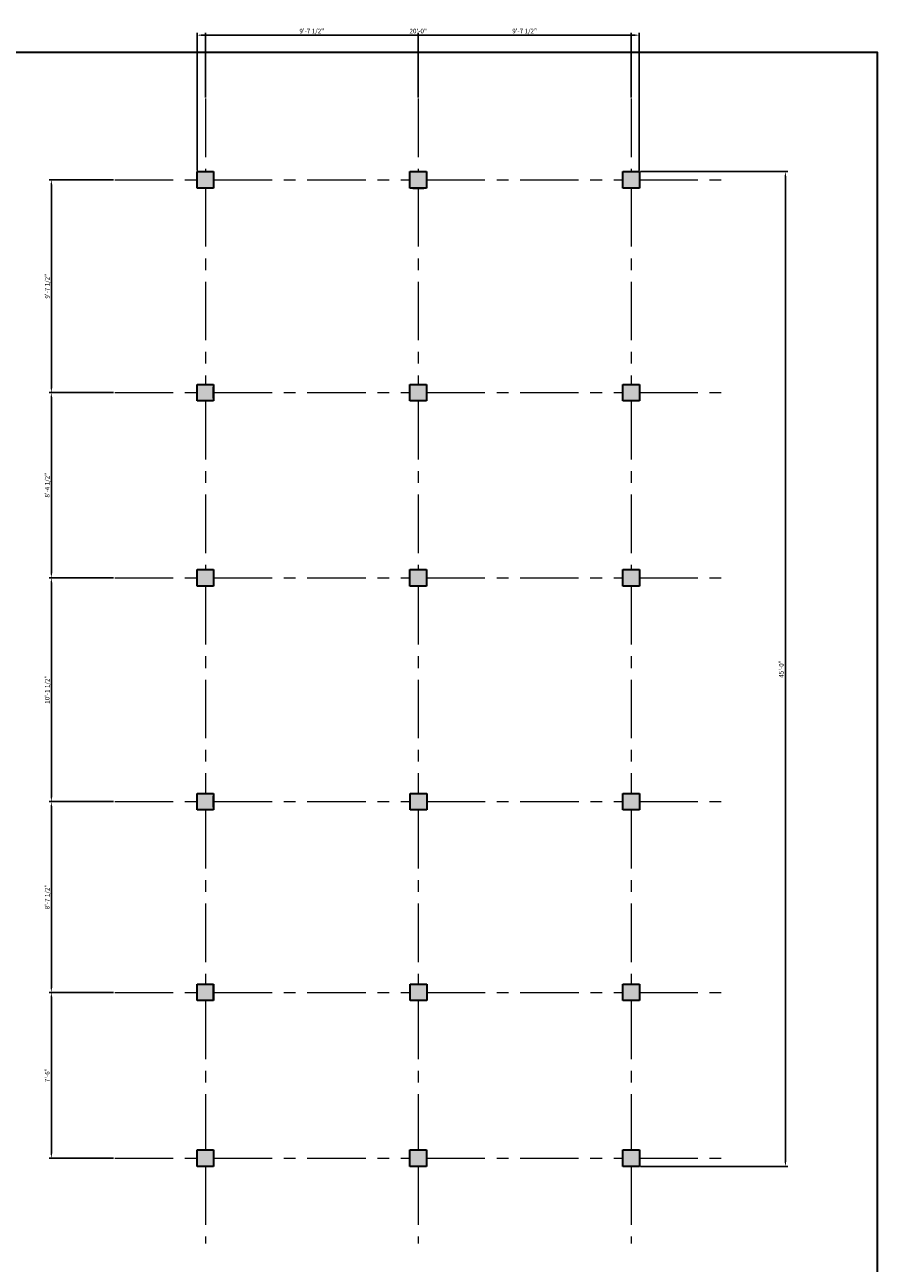
# Model space of a CAD drawing. Units: inches. Extents: x 2150 to 10686, y 1035 to 5077.
# Tile 12 of 12: x 10224 to 10686, y 1433 to 2106. Entities that reach past the tile are written whole.
import ezdxf

# ---------------------------------------------------------------- set-up
doc = ezdxf.new("R2010")
doc.units = ezdxf.units.IN
doc.linetypes.add('CENTER', pattern=[50.8, 31.75, -6.35, 6.35, -6.35])
for name, color, linetype, lineweight in [('A-ANNO-DIMS', 2, 'Continuous', 18), ('A-ANNO-TTLB', 7, 'Continuous', 35), ('A-COLS', 7, 'Continuous', 35), ('A-COLS-PATT', 8, 'Continuous', 13), ('A-GRID', 1, 'CENTER', 18)]:
    doc.layers.add(name, color=color, linetype=linetype, lineweight=lineweight)
doc.styles.get("Standard").update_dxf_attribs({"font": 'arial.ttf'})
doc.dimstyles.new('ISO-25', dxfattribs={"dimtxt": 2.5, "dimasz": 2.5, "dimexe": 1.25, "dimexo": 0.625, "dimtad": 1, "dimdec": 0, "dimlunit": 3, "dimtxsty": 'Standard', "dimcen": 2.5, "dimadec": 0, "dimazin": 0, "dimtfac": 1, "dimtdec": 0, "dimtmove": 0, "dimatfit": 3, "dimfxl": 1, "dimarcsym": 0})

# ---------------------------------------------------------------- blocks, each defined once
blk = doc.blocks.new('COL-SQUARE-9IN')
for p, q in [((0, 9), (9, 9)), ((0, 0), (0, 9)), ((9, 9), (9, 0)), ((9, 0), (0, 0))]:
    blk.add_line(p, q)
blk = doc.blocks.new('*D86')
at = {"layer": 'A-ANNO-DIMS', "color": 0, "lineweight": -2, "transparency": 16777216}
for p, q in [((10321.75, 2066.22), (10321.75, 2101.24)), ((10324.25, 2099.99), (10434.75, 2099.99)), ((10437.25, 2066.22), (10437.25, 2101.24))]:
    blk.add_line(p, q, dxfattribs=at)
at = {"layer": 'A-ANNO-DIMS', "color": 0, "transparency": 16777216}
for points in [[(10324.25, 2100.41), (10324.25, 2099.57), (10321.75, 2099.99)], [(10434.75, 2100.41), (10434.75, 2099.57), (10437.25, 2099.99)]]:
    blk.add_solid(points, dxfattribs=at)
at = {"layer": 'Defpoints', "color": 0, "transparency": 16777216}
for p in [(10437.25, 2099.99), (10321.75, 2065.59), (10437.25, 2065.59)]:
    blk.add_point(p, dxfattribs=at)
at = {"layer": 'A-ANNO-DIMS', "color": 0, "transparency": 16777216, "insert": (10379.5, 2101.91), "char_height": 2.5, "attachment_point": 5}
blk.add_mtext('9\'-7 1/2"', dxfattribs=at)
blk = doc.blocks.new('*D87')
at = {"layer": 'A-ANNO-DIMS', "color": 0, "lineweight": -2, "transparency": 16777216}
for p, q in [((10437.25, 2066.22), (10437.25, 2101.24)), ((10439.75, 2099.99), (10550.25, 2099.99)), ((10552.75, 2066.22), (10552.75, 2101.24))]:
    blk.add_line(p, q, dxfattribs=at)
at = {"layer": 'A-ANNO-DIMS', "color": 0, "transparency": 16777216}
for points in [[(10439.75, 2100.41), (10439.75, 2099.57), (10437.25, 2099.99)], [(10550.25, 2100.41), (10550.25, 2099.57), (10552.75, 2099.99)]]:
    blk.add_solid(points, dxfattribs=at)
at = {"layer": 'Defpoints', "color": 0, "transparency": 16777216}
for p in [(10552.75, 2099.99), (10437.25, 2065.59), (10552.75, 2065.59)]:
    blk.add_point(p, dxfattribs=at)
at = {"layer": 'A-ANNO-DIMS', "color": 0, "transparency": 16777216, "insert": (10495, 2101.91), "char_height": 2.5, "attachment_point": 5}
blk.add_mtext('9\'-7 1/2"', dxfattribs=at)
blk = doc.blocks.new('*D88')
at = {"layer": 'A-ANNO-DIMS', "color": 0, "lineweight": -2, "transparency": 16777216}
for p, q in [((10271.96, 2021.46), (10236.93, 2021.46)), ((10238.18, 2018.96), (10238.18, 1908.46)), ((10271.96, 1905.96), (10236.93, 1905.96))]:
    blk.add_line(p, q, dxfattribs=at)
at = {"layer": 'A-ANNO-DIMS', "color": 0, "transparency": 16777216}
for points in [[(10237.77, 2018.96), (10238.6, 2018.96), (10238.18, 2021.46)], [(10237.77, 1908.46), (10238.6, 1908.46), (10238.18, 1905.96)]]:
    blk.add_solid(points, dxfattribs=at)
at = {"layer": 'Defpoints', "color": 0, "transparency": 16777216}
for p in [(10272.58, 2021.46), (10238.18, 1905.96), (10272.58, 1905.96)]:
    blk.add_point(p, dxfattribs=at)
at = {"layer": 'A-ANNO-DIMS', "color": 0, "transparency": 16777216, "insert": (10236.26, 1963.71), "char_height": 2.5, "attachment_point": 5, "rotation": 90}
blk.add_mtext('9\'-7 1/2"', dxfattribs=at)
blk = doc.blocks.new('*D89')
at = {"layer": 'A-ANNO-DIMS', "color": 0, "lineweight": -2, "transparency": 16777216}
for p, q in [((10271.96, 1905.96), (10236.93, 1905.96)), ((10238.18, 1903.46), (10238.18, 1807.96)), ((10271.96, 1805.46), (10236.93, 1805.46))]:
    blk.add_line(p, q, dxfattribs=at)
at = {"layer": 'A-ANNO-DIMS', "color": 0, "transparency": 16777216}
for points in [[(10237.77, 1903.46), (10238.6, 1903.46), (10238.18, 1905.96)], [(10237.77, 1807.96), (10238.6, 1807.96), (10238.18, 1805.46)]]:
    blk.add_solid(points, dxfattribs=at)
at = {"layer": 'Defpoints', "color": 0, "transparency": 16777216}
for p in [(10272.58, 1905.96), (10238.18, 1805.46), (10272.58, 1805.46)]:
    blk.add_point(p, dxfattribs=at)
at = {"layer": 'A-ANNO-DIMS', "color": 0, "transparency": 16777216, "insert": (10236.26, 1855.71), "char_height": 2.5, "attachment_point": 5, "rotation": 90}
blk.add_mtext('8\'-4 1/2"', dxfattribs=at)
blk = doc.blocks.new('*D90')
at = {"layer": 'A-ANNO-DIMS', "color": 0, "lineweight": -2, "transparency": 16777216}
for p, q in [((10271.96, 1805.46), (10236.93, 1805.46)), ((10238.18, 1802.96), (10238.18, 1686.46)), ((10271.96, 1683.96), (10236.93, 1683.96))]:
    blk.add_line(p, q, dxfattribs=at)
at = {"layer": 'A-ANNO-DIMS', "color": 0, "transparency": 16777216}
for points in [[(10237.77, 1802.96), (10238.6, 1802.96), (10238.18, 1805.46)], [(10237.77, 1686.46), (10238.6, 1686.46), (10238.18, 1683.96)]]:
    blk.add_solid(points, dxfattribs=at)
at = {"layer": 'Defpoints', "color": 0, "transparency": 16777216}
for p in [(10272.58, 1805.46), (10238.18, 1683.96), (10272.58, 1683.96)]:
    blk.add_point(p, dxfattribs=at)
at = {"layer": 'A-ANNO-DIMS', "color": 0, "transparency": 16777216, "insert": (10236.26, 1744.71), "char_height": 2.5, "attachment_point": 5, "rotation": 90}
blk.add_mtext('10\'-1 1/2"', dxfattribs=at)
blk = doc.blocks.new('*D91')
at = {"layer": 'A-ANNO-DIMS', "color": 0, "lineweight": -2, "transparency": 16777216}
for p, q in [((10271.96, 1683.96), (10236.93, 1683.96)), ((10238.18, 1681.46), (10238.18, 1582.96)), ((10271.96, 1580.46), (10236.93, 1580.46))]:
    blk.add_line(p, q, dxfattribs=at)
at = {"layer": 'A-ANNO-DIMS', "color": 0, "transparency": 16777216}
for points in [[(10237.77, 1681.46), (10238.6, 1681.46), (10238.18, 1683.96)], [(10237.77, 1582.96), (10238.6, 1582.96), (10238.18, 1580.46)]]:
    blk.add_solid(points, dxfattribs=at)
at = {"layer": 'Defpoints', "color": 0, "transparency": 16777216}
for p in [(10272.58, 1683.96), (10238.18, 1580.46), (10272.58, 1580.46)]:
    blk.add_point(p, dxfattribs=at)
at = {"layer": 'A-ANNO-DIMS', "color": 0, "transparency": 16777216, "insert": (10236.26, 1632.21), "char_height": 2.5, "attachment_point": 5, "rotation": 90}
blk.add_mtext('8\'-7 1/2"', dxfattribs=at)
blk = doc.blocks.new('*D92')
at = {"layer": 'A-ANNO-DIMS', "color": 0, "lineweight": -2, "transparency": 16777216}
for p, q in [((10271.96, 1580.46), (10236.93, 1580.46)), ((10238.18, 1577.96), (10238.18, 1492.96)), ((10271.96, 1490.46), (10236.93, 1490.46))]:
    blk.add_line(p, q, dxfattribs=at)
at = {"layer": 'A-ANNO-DIMS', "color": 0, "transparency": 16777216}
for points in [[(10237.77, 1577.96), (10238.6, 1577.96), (10238.18, 1580.46)], [(10237.77, 1492.96), (10238.6, 1492.96), (10238.18, 1490.46)]]:
    blk.add_solid(points, dxfattribs=at)
at = {"layer": 'Defpoints', "color": 0, "transparency": 16777216}
for p in [(10272.58, 1580.46), (10238.18, 1490.46), (10272.58, 1490.46)]:
    blk.add_point(p, dxfattribs=at)
at = {"layer": 'A-ANNO-DIMS', "color": 0, "transparency": 16777216, "insert": (10236.28, 1535.46), "char_height": 2.5, "attachment_point": 5, "rotation": 90}
blk.add_mtext('7\'-6"', dxfattribs=at)
blk = doc.blocks.new('*D93')
at = {"layer": 'A-ANNO-DIMS', "color": 0, "lineweight": -2, "transparency": 16777216}
for p, q in [((10317.25, 2026.59), (10317.25, 2101.24)), ((10319.75, 2099.99), (10554.75, 2099.99)), ((10557.25, 2026.59), (10557.25, 2101.24))]:
    blk.add_line(p, q, dxfattribs=at)
at = {"layer": 'A-ANNO-DIMS', "color": 0, "transparency": 16777216}
for points in [[(10319.75, 2100.41), (10319.75, 2099.57), (10317.25, 2099.99)], [(10554.75, 2100.41), (10554.75, 2099.57), (10557.25, 2099.99)]]:
    blk.add_solid(points, dxfattribs=at)
at = {"layer": 'Defpoints', "color": 0, "transparency": 16777216}
for p in [(10557.25, 2099.99), (10317.25, 2025.96), (10557.25, 2025.96)]:
    blk.add_point(p, dxfattribs=at)
at = {"layer": 'A-ANNO-DIMS', "color": 0, "transparency": 16777216, "insert": (10437.25, 2101.89), "char_height": 2.5, "attachment_point": 5}
blk.add_mtext('20\'-0"', dxfattribs=at)
blk = doc.blocks.new('*D94')
at = {"layer": 'A-ANNO-DIMS', "color": 0, "lineweight": -2, "transparency": 16777216}
for p, q in [((10557.88, 2025.96), (10637.76, 2025.96)), ((10636.51, 1488.46), (10636.51, 2023.46)), ((10557.88, 1485.96), (10637.76, 1485.96))]:
    blk.add_line(p, q, dxfattribs=at)
at = {"layer": 'A-ANNO-DIMS', "color": 0, "transparency": 16777216}
for points in [[(10636.09, 2023.46), (10636.93, 2023.46), (10636.51, 2025.96)], [(10636.09, 1488.46), (10636.93, 1488.46), (10636.51, 1485.96)]]:
    blk.add_solid(points, dxfattribs=at)
at = {"layer": 'Defpoints', "color": 0, "transparency": 16777216}
for p in [(10557.25, 2025.96), (10636.51, 2025.96), (10557.25, 1485.96)]:
    blk.add_point(p, dxfattribs=at)
at = {"layer": 'A-ANNO-DIMS', "color": 0, "transparency": 16777216, "insert": (10634.61, 1755.96), "char_height": 2.5, "attachment_point": 5, "rotation": 90}
blk.add_mtext('45\'-0"', dxfattribs=at)

msp = doc.modelspace()

# ---------------------------------------------------------------- hatches: boundary and pattern name
at = {"layer": 'A-COLS-PATT'}
h = msp.add_hatch(color=256, dxfattribs=at)
h.dxf.hatch_style = 1
h.paths.add_polyline_path([(10326.25, 1494.96), (10317.25, 1494.96), (10317.25, 1485.96), (10326.25, 1485.96)])
h.paths.add_polyline_path([(10441.75, 1485.96), (10441.75, 1494.96), (10432.75, 1494.96), (10432.75, 1485.96)])
h.paths.add_polyline_path([(10557.25, 1485.96), (10557.25, 1494.96), (10548.25, 1494.96), (10548.25, 1485.96)])
h.paths.add_polyline_path([(10557.25, 1584.96), (10548.25, 1584.96), (10548.25, 1575.96), (10557.25, 1575.96)])
h.paths.add_polyline_path([(10432.85, 1575.96), (10441.85, 1575.96), (10441.85, 1584.96), (10432.85, 1584.96)])
h.paths.add_polyline_path([(10326.25, 1584.96), (10317.25, 1584.96), (10317.25, 1575.96), (10326.25, 1575.96)])
h.paths.add_polyline_path([(10326.25, 1688.46), (10317.25, 1688.46), (10317.25, 1679.46), (10326.25, 1679.46)])
h.paths.add_polyline_path([(10432.85, 1688.46), (10432.85, 1679.46), (10441.85, 1679.46), (10441.85, 1688.46)])
h.paths.add_polyline_path([(10557.25, 1688.46), (10548.25, 1688.46), (10548.25, 1679.46), (10557.25, 1679.46)])
h.paths.add_polyline_path([(10548.25, 1809.96), (10548.25, 1800.96), (10557.25, 1800.96), (10557.25, 1809.96)])
h.paths.add_polyline_path([(10432.75, 1809.96), (10432.75, 1800.96), (10441.75, 1800.96), (10441.75, 1809.96)])
h.paths.add_polyline_path([(10326.25, 1809.96), (10317.25, 1809.96), (10317.25, 1800.96), (10326.25, 1800.96)])
h.paths.add_polyline_path([(10317.25, 1910.46), (10317.25, 1901.46), (10326.25, 1901.46), (10326.25, 1910.46)])
h.paths.add_polyline_path([(10441.75, 1910.46), (10432.75, 1910.46), (10432.75, 1901.46), (10441.75, 1901.46)])
h.paths.add_polyline_path([(10548.25, 1910.46), (10548.25, 1901.46), (10557.25, 1901.46), (10557.25, 1910.46)])
h.paths.add_polyline_path([(10548.25, 2025.96), (10548.25, 2016.96), (10557.25, 2016.96), (10557.25, 2025.96)])
h.paths.add_polyline_path([(10441.75, 2025.96), (10432.75, 2025.96), (10432.75, 2016.96), (10441.75, 2016.96)])
h.paths.add_polyline_path([(10326.25, 2025.96), (10317.25, 2025.96), (10317.25, 2016.96), (10326.25, 2016.96)])

# ---------------------------------------------------------------- linework, layer by layer
at = {"layer": 'A-ANNO-TTLB'}
msp.add_lwpolyline([(9808.35, 2090.85), (10686.34, 2090.85), (10686.34, 1034.91), (9808.35, 1034.91)], close=True, dxfattribs=at)
at = {"layer": 'A-COLS'}
for p, q in [((10434.25, 2016.96), (10440.25, 2016.96)), ((10326.25, 1902.96), (10326.25, 1908.96)), ((10326.25, 1680.96), (10326.25, 1686.96)), ((10326.25, 1575.96), (10326.25, 1584.96))]:
    msp.add_line(p, q, dxfattribs=at)
at = {"layer": 'A-GRID'}
for p, q in [((10321.75, 2065.59), (10321.75, 2025.96)), ((10437.25, 2065.59), (10437.25, 2025.96)), ((10552.75, 2065.59), (10552.75, 2025.96)), ((10272.58, 2021.46), (10317.25, 2021.46)), ((10321.75, 2016.96), (10321.75, 1910.46)), ((10326.25, 2021.46), (10432.75, 2021.46)), ((10437.25, 2016.96), (10437.25, 1910.46)), ((10441.75, 2021.46), (10548.25, 2021.46)), ((10552.75, 2016.96), (10552.75, 1910.46)), ((10557.25, 2021.46), (10602.11, 2021.46)), ((10272.58, 1905.96), (10317.25, 1905.96)), ((10326.25, 1905.96), (10432.75, 1905.96)), ((10441.75, 1905.96), (10548.25, 1905.96)), ((10557.25, 1905.96), (10602.11, 1905.96)), ((10321.75, 1901.46), (10321.75, 1809.96)), ((10437.25, 1901.46), (10437.25, 1809.96)), ((10552.75, 1901.46), (10552.75, 1809.96)), ((10272.58, 1805.46), (10317.25, 1805.46)), ((10326.25, 1805.46), (10432.75, 1805.46)), ((10441.75, 1805.46), (10548.25, 1805.46)), ((10557.25, 1805.46), (10602.11, 1805.46)), ((10321.75, 1800.96), (10321.75, 1688.46)), ((10437.25, 1800.96), (10437.25, 1688.46)), ((10552.75, 1800.96), (10552.75, 1688.46)), ((10272.58, 1683.96), (10317.25, 1683.96)), ((10326.25, 1683.96), (10432.85, 1683.96)), ((10441.85, 1683.96), (10548.25, 1683.96)), ((10557.25, 1683.96), (10602.11, 1683.96)), ((10321.75, 1679.46), (10321.75, 1584.96)), ((10437.25, 1679.46), (10437.25, 1584.96)), ((10552.75, 1679.46), (10552.75, 1584.96)), ((10272.58, 1580.46), (10317.25, 1580.46)), ((10326.25, 1580.46), (10432.85, 1580.46)), ((10441.85, 1580.46), (10548.25, 1580.46)), ((10557.25, 1580.46), (10602.11, 1580.46)), ((10321.75, 1575.96), (10321.75, 1494.96)), ((10437.25, 1575.96), (10437.25, 1494.96)), ((10552.75, 1575.96), (10552.75, 1494.96)), ((10272.58, 1490.46), (10317.25, 1490.46)), ((10321.75, 1485.96), (10321.75, 1444.14)), ((10326.25, 1490.46), (10432.75, 1490.46)), ((10437.25, 1485.96), (10437.25, 1444.14)), ((10441.75, 1490.46), (10548.25, 1490.46)), ((10552.75, 1485.96), (10552.75, 1444.14)), ((10557.25, 1490.46), (10602.11, 1490.46))]:
    msp.add_line(p, q, dxfattribs=at)

# ---------------------------------------------------------------- block references
at = {"layer": 'A-COLS'}
for p in [(10317.26, 2016.96), (10432.76, 2016.96), (10548.26, 2016.96), (10317.26, 1901.46), (10432.76, 1901.46), (10548.26, 1901.46), (10317.26, 1800.96), (10432.76, 1800.96), (10548.26, 1800.96), (10317.26, 1679.46), (10432.85, 1679.46), (10548.26, 1679.46), (10317.26, 1575.96), (10432.85, 1575.96), (10548.26, 1575.96), (10317.26, 1485.96), (10432.76, 1485.96), (10548.26, 1485.96)]:
    msp.add_blockref('COL-SQUARE-9IN', p, dxfattribs=at)

# ---------------------------------------------------------------- dimensions: what is measured, and where the dimension line sits
at = {"layer": 'A-ANNO-DIMS'}
for base, p1, p2, picture, middle in [((10437.25, 2099.99), (10321.75, 2065.59), (10437.25, 2065.59), '*D86', (10379.5, 2101.91)), ((10552.75, 2099.99), (10437.25, 2065.59), (10552.75, 2065.59), '*D87', (10495, 2101.91)), ((10557.25, 2099.99), (10317.25, 2025.96), (10557.25, 2025.96), '*D93', (10437.25, 2101.89))]:
    dim = msp.add_linear_dim(base=base, p1=p1, p2=p2, dimstyle='ISO-25', override={"dimdec": 1, "dimlfac": 1, "dimrnd": 0, "dimzin": 1, "dimdsep": 46, "dimlunit": 4, "dimfrac": 2}, dxfattribs=at)
    dim.commit()
    dim.dimension.update_dxf_attribs({"geometry": picture, "text_midpoint": middle})
for base, p1, p2, picture, middle in [((10636.51, 2025.96), (10557.25, 1485.96), (10557.25, 2025.96), '*D94', (10634.61, 1755.96)), ((10238.18, 1905.96), (10272.58, 2021.46), (10272.58, 1905.96), '*D88', (10236.26, 1963.71)), ((10238.18, 1805.46), (10272.58, 1905.96), (10272.58, 1805.46), '*D89', (10236.26, 1855.71)), ((10238.18, 1683.96), (10272.58, 1805.46), (10272.58, 1683.96), '*D90', (10236.26, 1744.71)), ((10238.18, 1580.46), (10272.58, 1683.96), (10272.58, 1580.46), '*D91', (10236.26, 1632.21)), ((10238.18, 1490.46), (10272.58, 1580.46), (10272.58, 1490.46), '*D92', (10236.28, 1535.46))]:
    dim = msp.add_linear_dim(base=base, p1=p1, p2=p2, angle=90, dimstyle='ISO-25', override={"dimdec": 1, "dimlfac": 1, "dimrnd": 0, "dimzin": 1, "dimdsep": 46, "dimlunit": 4, "dimfrac": 2}, dxfattribs=at)
    dim.commit()
    dim.dimension.update_dxf_attribs({"geometry": picture, "text_midpoint": middle})

doc.saveas('drawing.dxf')
